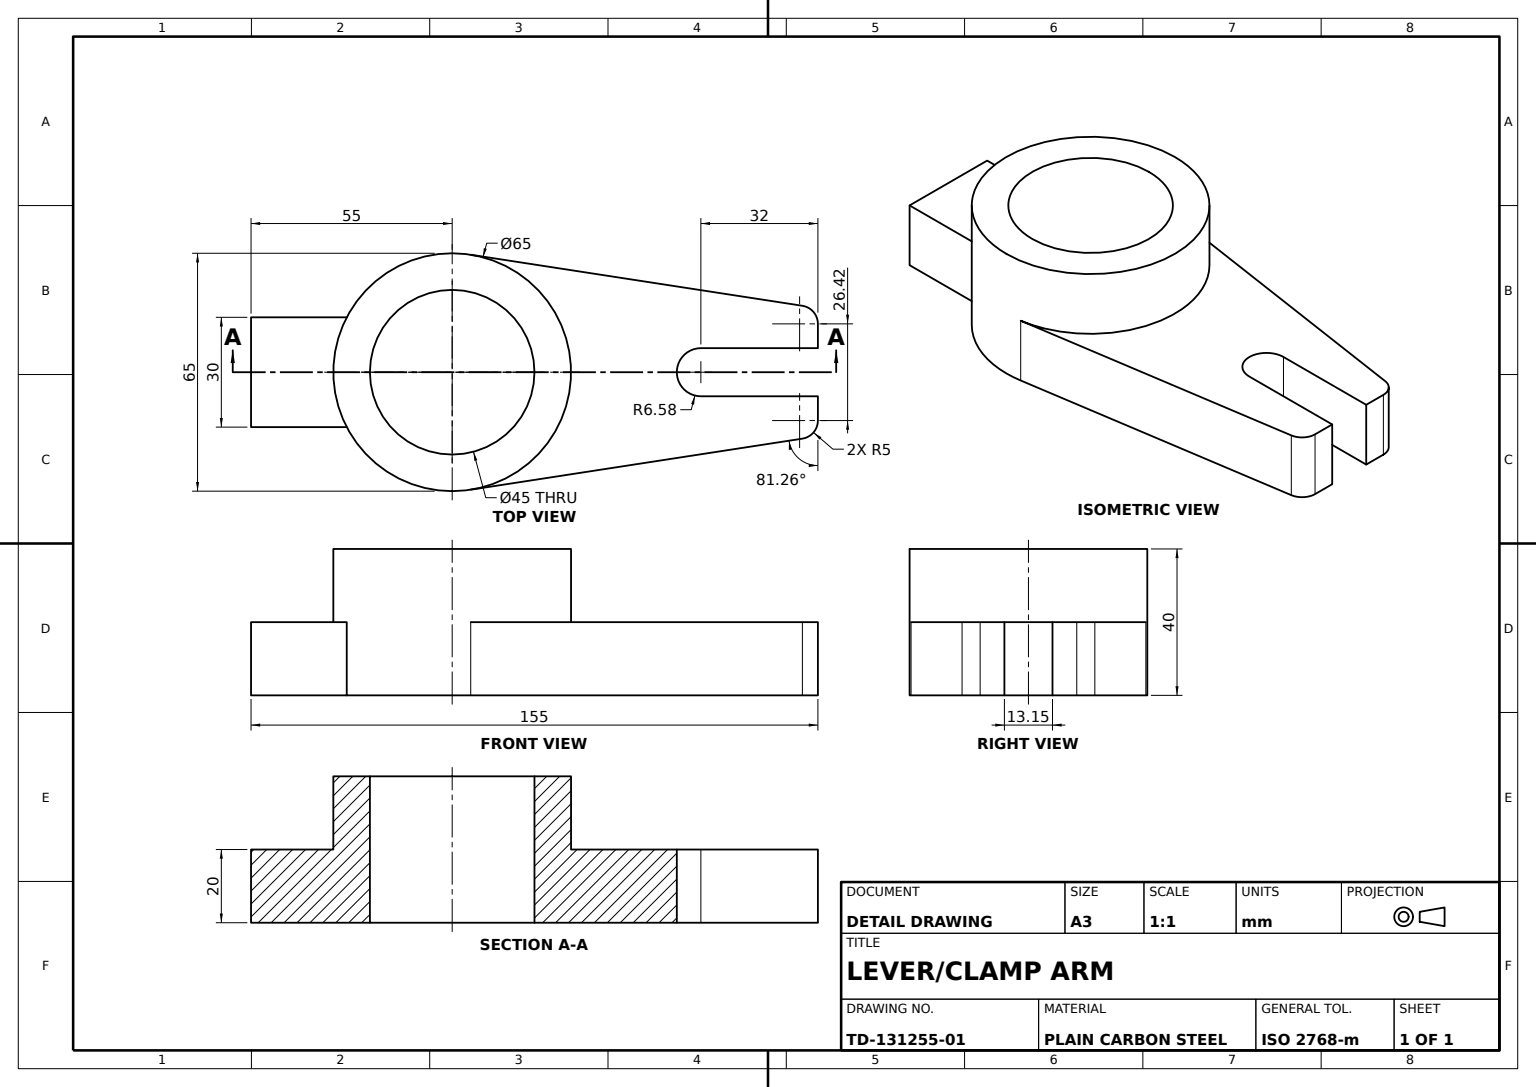
SolidWorks part; units mm, degrees
material "Plain Carbon Steel"
ref_plane "Front Plane" through (0, 0, 0) normal (0, 0, 1) x (1, 0, 0)
ref_plane "Top Plane" through (0, 0, 0) normal (0, 1, 0) x (1, 0, 0)
ref_plane "Right Plane" through (0, 0, 0) normal (1, 0, 0) x (0, 0, -1)
sketch "Hub Profile Ø65-Ø45" plane through (0, 0, 0) normal (0, 1, 0) x (1, 0, 0)
  circle A0 centre (0, 0) radius 32.5
  circle A1 centre (0, 0) radius 22.5
  dimension "D1" = 65
  dimension "D2" = 45
extrude "Hub Ø65 Bore Ø45" add sketch "Hub Profile Ø65-Ø45" along normal blind 40
ref_plane "Arm Sketch Plane" through (0, 0, 0) normal (0, 1, 0) x (1, 0, 0)
sketch "Fork Arm Profile" plane through (0, 0, 0) normal (0, 1, 0) x (1, 0, 0)
  line L1 (68, 6.5766) -> (100, 6.5766)
  line L2 (100, 6.5766) -> (100, 13.2103)
  line L3 (95.7602, 18.1522) -> (5.0678, 32.1024)
  line L5 (68, -6.5766) -> (100, -6.5766)
  line L6 (100, -6.5766) -> (100, -13.2103)
  line L7 (95.7602, -18.1522) -> (5.0678, -32.1024)
  arc A0 (68, 6.5766) -> (68, -6.5766) centre (68, 0) ccw
  arc A2 (95.7602, -18.1522) -> (100, -13.2103) centre (95, -13.2103) ccw
  arc A3 (100, 13.2103) -> (95.7602, 18.1522) centre (95, 13.2103) ccw
  arc A4 (5.0678, -32.1024) -> (5.0678, 32.1024) centre (0, 0) ccw
  point P15 (100, -17.5)
  point P18 (100, 17.5)
  dimension "D4" = 5
  dimension "D5" = 32.5
  dimension "D1" = 35
  dimension "D2" = 32
  dimension "D3" = 13.1532
  dimension "D6" = 4.2398
  dimension "D7" = 94.9322
extrude "Fork Arm" add sketch "Fork Arm Profile" along normal blind 20
sketch "Rear Block Profile 30x55" plane through (0, 0, 0) normal (0, 1, 0) x (1, 0, 0)
  line L1 (-55, -15) -> (-55, 15)
  line L2 (-55, 15) -> (-28.8314, 15)
  line L4 (-28.8314, -15) -> (-55, -15)
  arc A0 (-28.8314, 15) -> (-28.8314, -15) centre (0, 0) ccw
  point P6 (-55, 0)
  dimension "D3" = 32.5
  dimension "D1" = 30
  dimension "D2" = 55
extrude "Rear Block" add sketch "Rear Block Profile 30x55" along normal blind 20
